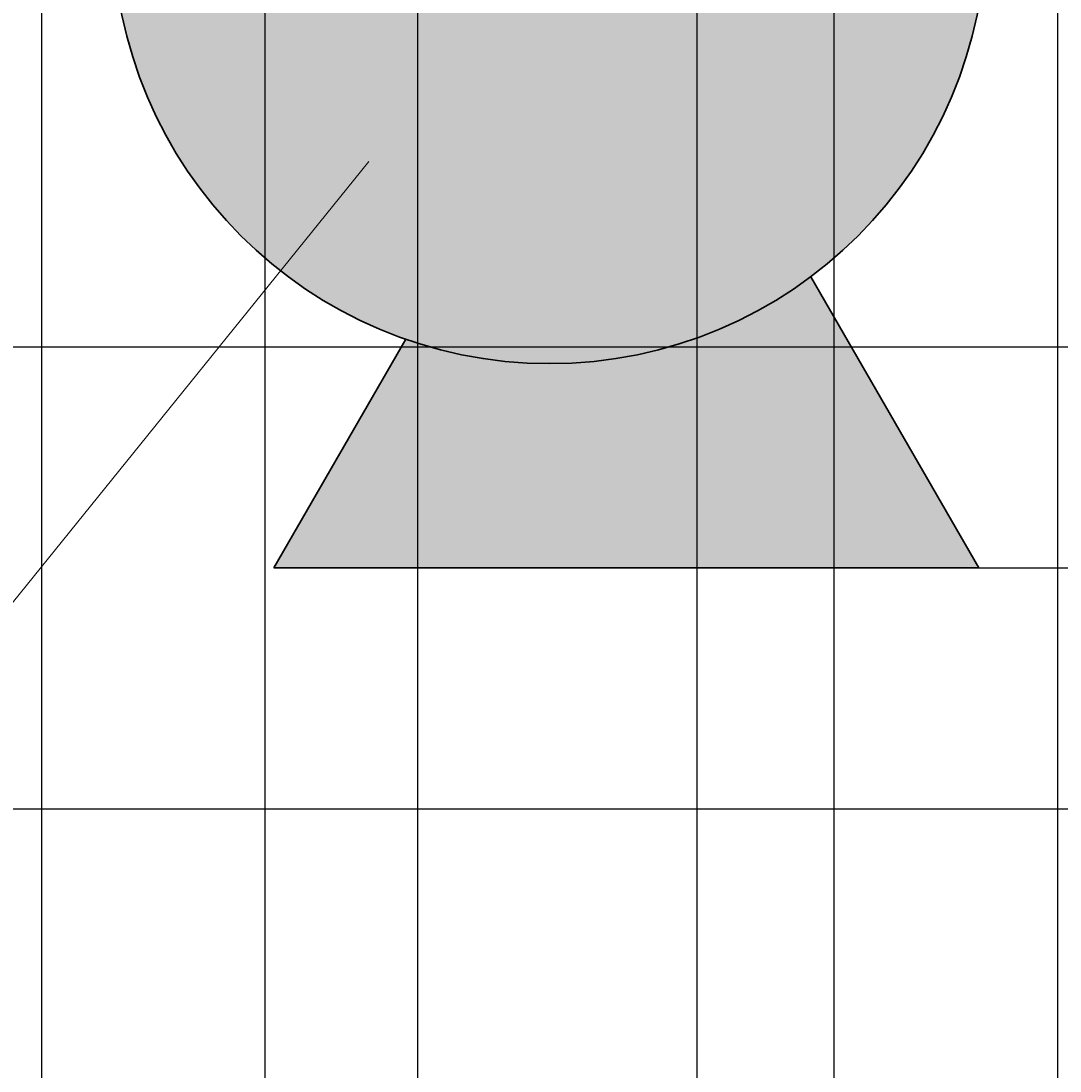
# Model space of a CAD drawing. Units: inches. Extents: x -1 to 292, y -3 to 199.
# Tile 36 of 52: x 232.46 to 254.96, y 19.84 to 42.57. Entities that reach past the tile are written whole.
import ezdxf

# ---------------------------------------------------------------- set-up
doc = ezdxf.new("R2010")
doc.units = ezdxf.units.IN
doc.header["$MEASUREMENT"] = 0
for name, color, linetype, lineweight in [('M-ANNO-LEAD', 2, 'Continuous', 18), ('M-DIMS', 2, 'Continuous', 18), ('M-EQPM', 7, 'Continuous', 35), ('M-PATT', 8, 'Continuous', 13)]:
    doc.layers.add(name, color=color, linetype=linetype, lineweight=lineweight)
doc.styles.get("Standard").update_dxf_attribs({"font": 'arial.ttf'})
doc.dimstyles.get("Standard").update_dxf_attribs({"dimtxt": 0.18, "dimasz": 0.18, "dimexe": 0.18, "dimexo": 0.0625, "dimgap": 0.09, "dimtad": 0, "dimtih": 1, "dimtoh": 1, "dimdec": 4, "dimzin": 0, "dimdsep": 46, "dimtxsty": 'Standard', "dimcen": 0.09, "dimadec": 0, "dimazin": 0, "dimtfac": 1, "dimtdec": 4, "dimtofl": 0, "dimtmove": 0, "dimatfit": 3, "dimfxl": 1, "dimtolj": 1, "dimtzin": 0, "dimarcsym": 0})

# ---------------------------------------------------------------- blocks, each defined once
blk = doc.blocks.new('*D11')
at = {"layer": 'Defpoints', "color": 0, "transparency": 16777216}
for p in [(79.013, 35.514), (292.04, 35.514), (79.013, 25.514)]:
    blk.add_point(p, dxfattribs=at)
at = {"layer": 'M-DIMS', "color": 0, "lineweight": -2, "transparency": 16777216}
for p, q in [((79.076, 35.514), (292.22, 35.514)), ((292.04, 35.334), (292.04, 30.696)), ((292.04, 25.694), (292.04, 30.332)), ((79.076, 25.514), (292.22, 25.514))]:
    blk.add_line(p, q, dxfattribs=at)
at = {"layer": 'M-DIMS', "color": 0, "transparency": 16777216}
for points in [[(292.01, 35.334), (292.07, 35.334), (292.04, 35.514)], [(292.01, 25.694), (292.07, 25.694), (292.04, 25.514)]]:
    blk.add_solid(points, dxfattribs=at)
at = {"layer": 'M-DIMS', "color": 0, "transparency": 16777216, "insert": (292.04, 30.514), "char_height": 0.18, "attachment_point": 5}
blk.add_mtext('\\A1;10', dxfattribs=at)
blk = doc.blocks.new('*D25')
at = {"layer": 'Defpoints', "color": 0, "transparency": 16777216}
for p in [(273.066, 88.419), (215.241, 88.13), (273.066, -2.71)]:
    blk.add_point(p, dxfattribs=at)
at = {"layer": 'M-DIMS', "color": 0, "lineweight": -2, "transparency": 16777216}
for p, q in [((273.066, 88.357), (273.066, -2.89)), ((215.241, 88.068), (215.241, -2.89)), ((215.421, -2.71), (243.76, -2.71)), ((272.886, -2.71), (244.547, -2.71))]:
    blk.add_line(p, q, dxfattribs=at)
at = {"layer": 'M-DIMS', "color": 0, "transparency": 16777216}
for points in [[(215.421, -2.68), (215.421, -2.74), (215.241, -2.71)], [(272.886, -2.68), (272.886, -2.74), (273.066, -2.71)]]:
    blk.add_solid(points, dxfattribs=at)
at = {"layer": 'M-DIMS', "color": 0, "transparency": 16777216, "insert": (244.153, -2.71), "char_height": 0.18, "attachment_point": 5}
blk.add_mtext('\\A1;57.83', dxfattribs=at)
blk = doc.blocks.new('*D28')
at = {"layer": 'Defpoints', "color": 0, "transparency": 16777216}
for p in [(241.044, 80.582), (247.095, 80.582), (247.095, -2.71)]:
    blk.add_point(p, dxfattribs=at)
at = {"layer": 'M-DIMS', "color": 0, "lineweight": -2, "transparency": 16777216}
for p, q in [((241.044, 80.52), (241.044, -2.89)), ((247.095, 80.52), (247.095, -2.89)), ((241.224, -2.71), (243.692, -2.71)), ((246.915, -2.71), (244.446, -2.71))]:
    blk.add_line(p, q, dxfattribs=at)
at = {"layer": 'M-DIMS', "color": 0, "transparency": 16777216}
for points in [[(241.224, -2.68), (241.224, -2.74), (241.044, -2.71)], [(246.915, -2.68), (246.915, -2.74), (247.095, -2.71)]]:
    blk.add_solid(points, dxfattribs=at)
at = {"layer": 'M-DIMS', "color": 0, "transparency": 16777216, "insert": (244.069, -2.71), "char_height": 0.18, "attachment_point": 5}
blk.add_mtext('\\A1;6.051', dxfattribs=at)
blk = doc.blocks.new('*D30')
at = {"layer": 'Defpoints', "color": 0, "transparency": 16777216}
for p in [(232.903, 62.582), (254.903, 62.582), (254.903, -2.71)]:
    blk.add_point(p, dxfattribs=at)
at = {"layer": 'M-DIMS', "color": 0, "lineweight": -2, "transparency": 16777216}
for p, q in [((232.903, 62.52), (232.903, -2.89)), ((254.903, 62.52), (254.903, -2.89)), ((233.083, -2.71), (243.684, -2.71)), ((254.723, -2.71), (244.123, -2.71))]:
    blk.add_line(p, q, dxfattribs=at)
at = {"layer": 'M-DIMS', "color": 0, "transparency": 16777216}
for points in [[(233.083, -2.68), (233.083, -2.74), (232.903, -2.71)], [(254.723, -2.68), (254.723, -2.74), (254.903, -2.71)]]:
    blk.add_solid(points, dxfattribs=at)
at = {"layer": 'M-DIMS', "color": 0, "transparency": 16777216, "insert": (243.903, -2.71), "char_height": 0.18, "attachment_point": 5}
blk.add_mtext('\\A1;22', dxfattribs=at)
blk = doc.blocks.new('*D32')
at = {"layer": 'Defpoints', "color": 0, "transparency": 16777216}
for p in [(237.744, 67.423), (250.063, 67.423), (250.063, -2.71)]:
    blk.add_point(p, dxfattribs=at)
at = {"layer": 'M-DIMS', "color": 0, "lineweight": -2, "transparency": 16777216}
for p, q in [((237.744, 67.36), (237.744, -2.89)), ((250.063, 67.36), (250.063, -2.89)), ((237.924, -2.71), (243.448, -2.71)), ((249.883, -2.71), (244.359, -2.71))]:
    blk.add_line(p, q, dxfattribs=at)
at = {"layer": 'M-DIMS', "color": 0, "transparency": 16777216}
for points in [[(237.924, -2.68), (237.924, -2.74), (237.744, -2.71)], [(249.883, -2.68), (249.883, -2.74), (250.063, -2.71)]]:
    blk.add_solid(points, dxfattribs=at)
at = {"layer": 'M-DIMS', "color": 0, "transparency": 16777216, "insert": (243.903, -2.71), "char_height": 0.18, "attachment_point": 5}
blk.add_mtext('\\A1;12.319', dxfattribs=at)
blk = doc.blocks.new('*D33')
at = {"layer": 'Defpoints', "color": 0, "transparency": 16777216}
for p in [(242.955, 125.727), (292.04, 125.727), (237.933, 30.73)]:
    blk.add_point(p, dxfattribs=at)
at = {"layer": 'M-DIMS', "color": 0, "lineweight": -2, "transparency": 16777216}
for p, q in [((243.018, 125.727), (292.22, 125.727)), ((292.04, 125.547), (292.04, 78.41)), ((292.04, 30.91), (292.04, 78.046)), ((237.996, 30.73), (292.22, 30.73))]:
    blk.add_line(p, q, dxfattribs=at)
at = {"layer": 'M-DIMS', "color": 0, "transparency": 16777216}
for points in [[(292.01, 125.547), (292.07, 125.547), (292.04, 125.727)], [(292.01, 30.91), (292.07, 30.91), (292.04, 30.73)]]:
    blk.add_solid(points, dxfattribs=at)
at = {"layer": 'M-DIMS', "color": 0, "transparency": 16777216, "insert": (292.04, 78.228), "char_height": 0.18, "attachment_point": 5}
blk.add_mtext('\\A1;95', dxfattribs=at)

msp = doc.modelspace()

# ---------------------------------------------------------------- hatches: boundary and pattern name
at = {"layer": 'M-PATT'}
h = msp.add_hatch(color=256, dxfattribs=at)
h.set_gradient(color1=(0, 255, 255), color2=(0, 255, 255), tint=1, name='CYLINDER')
h.paths.add_polyline_path([(256.8092, 99.5764), (256.4077, 99.3157), (253.7155, 100.87), (251.3221, 99.3157), (248.6299, 100.87), (246.2365, 99.3157), (243.5443, 100.87), (241.1509, 99.3157), (238.4587, 100.87), (236.4209, 99.5466), (236.4209, 97.1861), (234.9209, 97.1861), (234.9209, 99.9764), (233.3731, 100.87), (230.9797, 99.3157, 1.0704128)])
h.paths.add_polyline_path([(234.4549, 44.5975, 1), (253.3518, 44.5975, 1)])
h.paths.add_polyline_path([(235.4822, 48.8821), (220.034, 57.8011), (220.034, 85.363), (232.4507, 92.5318, -0.0853739), (231.0925, 96.7051), (215.7407, 87.8418), (215.7407, 55.3224), (234.4552, 44.5176, -0.0021162), (234.4549, 44.5975, -0.1182098)])
h.paths.add_polyline_path([(222.7904, 52.8755), (221.8492, 54.5058), (223.7904, 54.6075)], flags=16)
h.paths.add_polyline_path([(216.828, 66.8912), (217.7692, 68.5216), (218.828, 66.8912)], flags=16)
h.paths.add_polyline_path([(216.8084, 83.826), (217.7497, 85.4564), (218.8084, 83.826)], flags=16)
h.paths.add_polyline_path([(226.468, 92.8803), (228.3442, 93.0348), (227.6068, 91.2362)], flags=16)
h.paths.add_polyline_path([(272.5659, 88.1304), (260.2765, 95.2257), (259.0113, 93.0196), (263.0639, 91.1046), (263.4912, 92.0087), (264.5631, 90.4612), (262.6367, 90.2004), (263.0639, 91.1046), (259.0113, 93.0196), (257.8918, 91.0677), (267.7726, 85.363), (267.7726, 57.8011), (255.5043, 50.718), (257.0663, 46.085), (272.5659, 55.0337)])
h.paths.add_polyline_path([(263.6286, 51.5636), (261.7461, 51.5636), (262.6286, 53.2956)], flags=16)
h.paths.add_polyline_path([(269.8773, 65.3608), (268.8186, 66.9911), (270.8186, 66.9911)], flags=16)
h.paths.add_polyline_path([(269.8773, 80.8843), (268.8186, 82.5146), (270.8186, 82.5146)], flags=16)
h.paths.add_polyline_path([(255.5043, 50.718), (252.3244, 48.8821, -0.1182098), (253.3518, 44.5975, -0.0177685), (253.3279, 43.9266), (257.0663, 46.085)])
h.paths.add_polyline_path([(260.2765, 95.2257), (256.7809, 97.2439, -0.0959457), (255.356, 92.5318), (257.8918, 91.0677)])
h = msp.add_hatch(color=256, dxfattribs=at)
h.set_gradient(color1=(128, 128, 128), color2=(192, 192, 192), tint=1, name='CYLINDER')
h.paths.add_polyline_path([(158.4295, 25.5141), (158.4295, 35.5141), (148.4295, 35.5141), (148.4295, 25.5141)])
h.paths.add_polyline_path([(79.013, 25.5141), (79.013, 35.5141), (69.013, 35.5141), (69.013, 25.5141)])
h.paths.add_polyline_path([(253.2006, 30.7296), (249.5623, 37.0313, -0.2494892), (240.7896, 35.6769), (237.9333, 30.7296)])

# ---------------------------------------------------------------- linework, layer by layer
at = {"layer": 'M-ANNO-LEAD'}
msp.add_line((239.9895, 39.5261), (217.6733, 11.8896), dxfattribs=at)
at = {"layer": 'M-EQPM'}
for p, q in [((253.2006, 30.7296), (249.5623, 37.0313)), ((237.9333, 30.7296), (240.7896, 35.6769)), ((237.9333, 30.7296), (253.2006, 30.7296))]:
    msp.add_line(p, q, dxfattribs=at)
msp.add_circle((243.9033, 44.5975), 9.4484, dxfattribs=at)

# ---------------------------------------------------------------- dimensions: what is measured, and where the dimension line sits
at = {"layer": 'M-DIMS'}
for base, p1, p2, picture, middle in [((292.0399, 125.7269), (237.9333, 30.7296), (242.9552, 125.7269), '*D33', (292.0399, 78.2282)), ((292.0399, 35.5141), (79.013, 25.5141), (79.013, 35.5141), '*D11', (292.0399, 30.5141))]:
    dim = msp.add_linear_dim(base=base, p1=p1, p2=p2, angle=90, dimstyle='Standard', override={"dimdec": 0, "dimlfac": 1, "dimrnd": 0, "dimzin": 0, "dimdsep": 46, "dimlunit": 2}, dxfattribs=at)
    dim.commit()
    dim.dimension.update_dxf_attribs({"geometry": picture, "text_midpoint": middle})
for base, p1, p2, override, picture, middle in [((273.0659, -2.7104), (215.2407, 88.1304), (273.0659, 88.4191), {"dimdec": 2, "dimlfac": 1, "dimrnd": 0, "dimzin": 0, "dimdsep": 46, "dimlunit": 2}, '*D25', (244.1533, -2.7104)), ((247.0947, -2.7104), (241.0437, 80.5821), (247.0947, 80.5821), {"dimdec": 3, "dimlfac": 1, "dimrnd": 0, "dimzin": 0, "dimdsep": 46, "dimlunit": 2}, '*D28', (244.0692, -2.7104)), ((250.0626, -2.7104), (237.744, 67.4228), (250.0626, 67.4228), {"dimdec": 3, "dimlfac": 1, "dimrnd": 0, "dimzin": 0, "dimdsep": 46, "dimlunit": 2}, '*D32', (243.9033, -2.7104)), ((254.9033, -2.7104), (232.9033, 62.5821), (254.9033, 62.5821), {"dimdec": 0, "dimlfac": 1, "dimrnd": 0, "dimzin": 0, "dimdsep": 46, "dimlunit": 2}, '*D30', (243.9033, -2.7104))]:
    dim = msp.add_linear_dim(base=base, p1=p1, p2=p2, dimstyle='Standard', override=override, dxfattribs=at)
    dim.commit()
    dim.dimension.update_dxf_attribs({"geometry": picture, "text_midpoint": middle})

doc.saveas('drawing.dxf')
